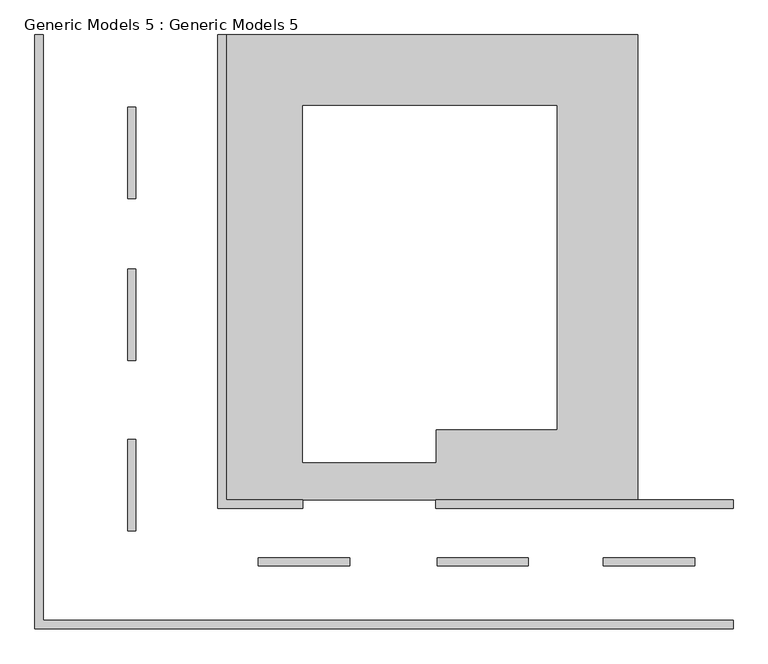
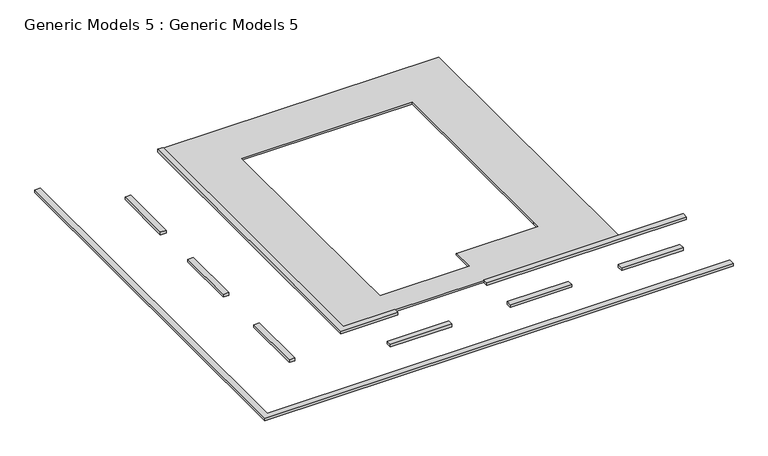
"""IFC4 building model written with IfcOpenShell, lengths in millimetres: proxy geometry, Generic Models 5 : Generic Models 5."""

from ifc_helpers import new_model, si_unit, frame, origin, place, context, project, spatial, polyline, outline, extrude, source, transform, mapped, element, save


def generic_models_5_generic_models_5_f3326099(model_context):
    return source(origin(), model_context, "Body", "SweptSolid", [
        extrude(outline(polyline([(-15594.5519188, 8152.7632107), (-15594.5519188, 4799.9632107), (-15899.3519188, 4799.9632107), (-15899.3519188, 8152.7632107), (-15594.5519188, 8152.7632107)])), frame((0.0, 0.0, -304.8), z_axis=(0.0, 0.0, 1.0), x_axis=(1.0, 0.0, 0.0)), (0.0, 0.0, 1.0), 159.1005775),
        extrude(outline(polyline([(-15594.5519188, 2209.1632107), (-15594.5519188, -1143.6367893), (-15899.3519188, -1143.6367893), (-15899.3519188, 2209.1632107), (-15594.5519188, 2209.1632107)])), frame((0.0, 0.0, -304.8), z_axis=(0.0, 0.0, 1.0), x_axis=(1.0, 0.0, 0.0)), (0.0, 0.0, 1.0), 159.1005775),
        extrude(outline(polyline([(-15594.5519188, -4039.2367893), (-15594.5519188, -7392.0367893), (-15899.3519188, -7392.0367893), (-15899.3519188, -4039.2367893), (-15594.5519188, -4039.2367893)])), frame((0.0, 0.0, -304.8), z_axis=(0.0, 0.0, 1.0), x_axis=(1.0, 0.0, 0.0)), (0.0, 0.0, 1.0), 159.1005775),
        extrude(outline(polyline([(-7753.7025595, -8680.4793248), (-11106.5025595, -8680.4793248), (-11106.5025595, -8375.6793248), (-7753.7025595, -8375.6793248), (-7753.7025595, -8680.4793248)])), frame((0.0, 0.0, -304.8), z_axis=(0.0, 0.0, 1.0), x_axis=(1.0, 0.0, 0.0)), (0.0, 0.0, 1.0), 159.1005775),
        extrude(outline(polyline([(-1200.5025595, -8680.4793248), (-4553.3025595, -8680.4793248), (-4553.3025595, -8375.6793248), (-1200.5025595, -8375.6793248), (-1200.5025595, -8680.4793248)])), frame((0.0, 0.0, -304.8), z_axis=(0.0, 0.0, 1.0), x_axis=(1.0, 0.0, 0.0)), (0.0, 0.0, 1.0), 159.1005775),
        extrude(outline(polyline([(4895.4974405, -8680.4793248), (1542.6974405, -8680.4793248), (1542.6974405, -8375.6793248), (4895.4974405, -8375.6793248), (4895.4974405, -8680.4793248)])), frame((0.0, 0.0, -304.8), z_axis=(0.0, 0.0, 1.0), x_axis=(1.0, 0.0, 0.0)), (0.0, 0.0, 1.0), 159.1005775),
        extrude(outline(polyline([(-9480.9025595, -6260.4117016), (-9480.9025595, -6565.2117016), (-12593.5524046, -6565.2117016), (-12593.5524046, 10808.3882984), (-12288.7524046, 10808.3882984), (-12288.7524046, -6260.4117016), (-9480.9025595, -6260.4117016)])), frame((0.0, 0.0, -304.8), z_axis=(0.0, 0.0, 1.0), x_axis=(1.0, 0.0, 0.0)), (0.0, 0.0, 1.0), 154.4641193),
        extrude(outline(polyline([(-19299.1524046, -10984.8117016), (-19299.1524046, 10808.3882984), (-18994.3524046, 10808.3882984), (-18994.3524046, -10680.0117016), (6304.0475954, -10680.0117016), (6304.0475954, -10984.8117016), (-19299.1524046, -10984.8117016)])), frame((0.0, 0.0, -304.8), z_axis=(0.0, 0.0, 1.0), x_axis=(1.0, 0.0, 0.0)), (0.0, 0.0, 1.0), 154.4641193),
        extrude(outline(polyline([(-4604.1025595, -6565.2117016), (-4604.1025595, -6260.4117016), (6304.0475954, -6260.4117016), (6304.0475954, -6565.2117016), (-4604.1025595, -6565.2117016)])), frame((0.0, 0.0, -304.8), z_axis=(0.0, 0.0, 1.0), x_axis=(1.0, 0.0, 0.0)), (0.0, 0.0, 1.0), 154.4641193),
        extrude(outline(polyline([(2798.8475954, 10808.3882984), (2798.8475954, -6260.4117016), (-12288.7524046, -6260.4117016), (-12288.7524046, 10808.3882984), (2798.8475954, 10808.3882984)]), holes=[polyline([(-165.4525595, 8209.9132107), (-9480.9025595, 8209.9132107), (-9480.9025595, -3239.1367893), (-9480.9025595, -4883.7867893), (-4604.1025595, -4883.7867893), (-4604.1025595, -3664.5867893), (-165.4525595, -3664.5867893), (-165.4525595, -3239.1367893), (-165.4525595, 8209.9132107)])]), frame((0.0, 0.0, -304.8), z_axis=(0.0, 0.0, 1.0), x_axis=(1.0, 0.0, 0.0)), (0.0, 0.0, 1.0), 108.6007587),
    ])


if __name__ == "__main__":
    model = new_model("IFC4")
    model_context = context("Model", 3, world=origin())
    ifc_project = project(units=[si_unit("LENGTHUNIT", "METRE", prefix="MILLI")], contexts=[model_context])
    site = spatial("IfcSite", under=ifc_project)
    building = spatial("IfcBuilding", under=site)
    placement = place(None, origin())
    generic_models_5_generic_models_5_shape = generic_models_5_generic_models_5_f3326099(model_context)
    element("IfcBuildingElementProxy", 1, Name="Generic Models 5 : Generic Models 5", ObjectType="Generic Models 5 : Generic Models 5", at=placement, inside=building, context=model_context, shape_type="MappedRepresentation", body=[
        mapped(generic_models_5_generic_models_5_shape, transform((0.0, 0.0, 0.0), x_axis=(1.0, 0.0, 0.0), y_axis=(0.0, 1.0, 0.0), z_axis=(0.0, 0.0, 1.0))),
    ])
    save(model, "model.ifc")

# Revit data of these elements
# Element 1 (IfcBuildingElementProxy, "Generic Models 5 : Generic Models 5")
#   Materials on its faces: "Gypsum Wall Board"
# Materials
#   "Gypsum Wall Board": class "Generic", colour RGB 228 228 228, transparency 0, Description = "Gypsum Wall Board", Cost = 0
